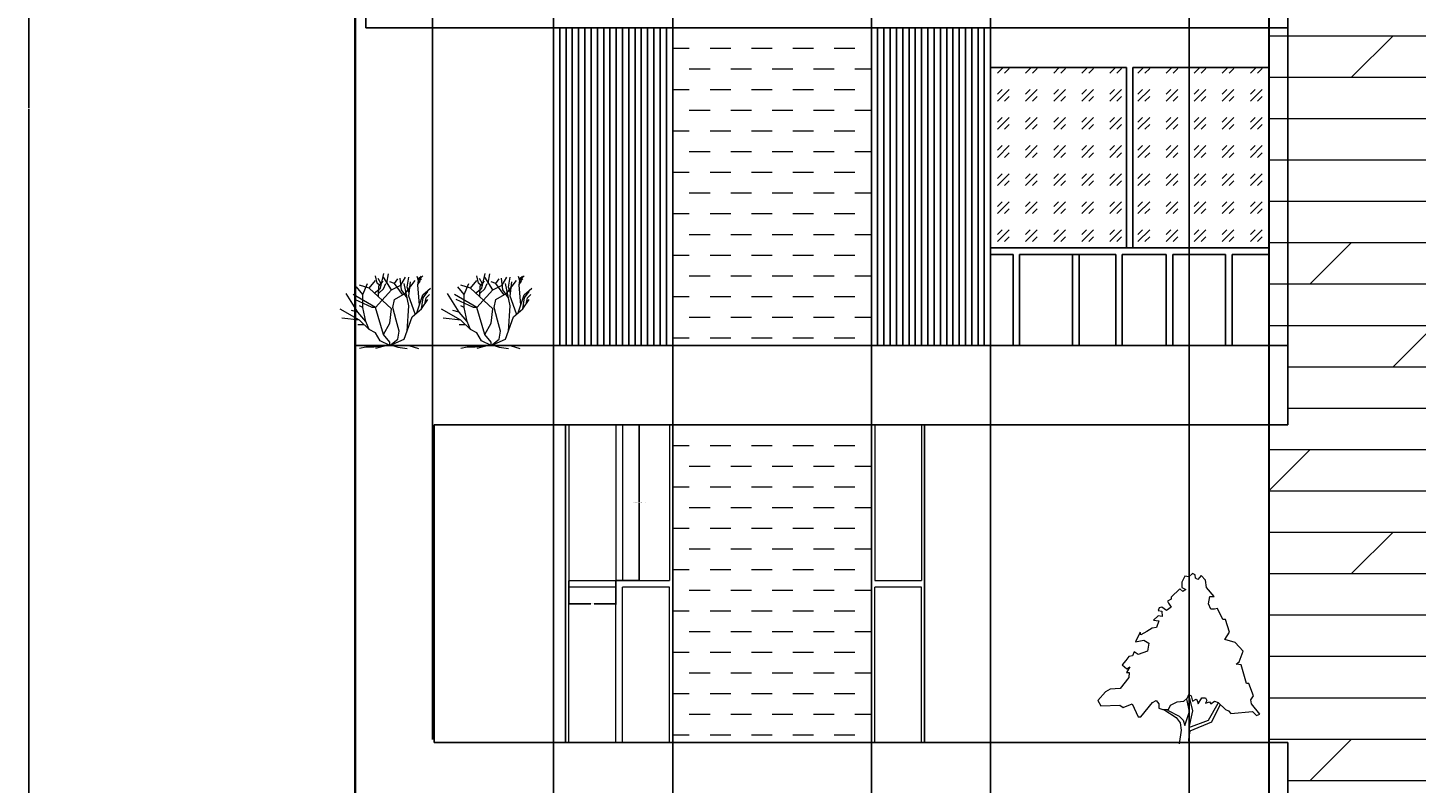
# Model space of a CAD drawing. Units: inches. Extents: x 250 to 1217, y -42 to 832.
# Tile 2 of 7: x 250 to 670, y 187 to 415. Entities that reach past the tile are written whole.
import ezdxf

# ---------------------------------------------------------------- set-up
doc = ezdxf.new("R2010")
doc.units = ezdxf.units.IN
doc.header["$MEASUREMENT"] = 0
for name, color, linetype, lineweight in [('A-ANNO-DIMS', 2, 'Continuous', 18), ('A-ELEV', 7, 'Continuous', 25), ('A-ELEV-PATT', 8, 'Continuous', 13), ('A-GLAZ', 4, 'Continuous', 18), ('L-PLNT', 3, 'Continuous', 13)]:
    doc.layers.add(name, color=color, linetype=linetype, lineweight=lineweight)
doc.styles.get("Standard").update_dxf_attribs({"font": 'arial.ttf'})
doc.dimstyles.get("Standard").update_dxf_attribs({"dimtxt": 0.18, "dimasz": 0.18, "dimexe": 0.18, "dimexo": 0.0625, "dimgap": 0.09, "dimtad": 0, "dimtih": 1, "dimtoh": 1, "dimdec": 4, "dimzin": 0, "dimdsep": 46, "dimtxsty": 'Standard', "dimcen": 0.09, "dimadec": 0, "dimazin": 0, "dimtfac": 1, "dimtdec": 4, "dimtofl": 0, "dimtmove": 0, "dimatfit": 3, "dimfxl": 1, "dimtolj": 1, "dimtzin": 0, "dimarcsym": 0})

# ---------------------------------------------------------------- blocks, each defined once
blk = doc.blocks.new('*U3')
for points in [[(22.0124, 137.721), (18.5475, 141.5624), (15.5282, 138.2446), (13.8028, 139.3505), (13.3714, 142.1153), (11.2148, 143.2214), (8.1954, 140.4564), (4.7447, 141.0094), (2.1567, 136.0326), (2.1567, 131.6088), (5.6074, 129.9499), (3.0193, 128.2909), (0.4313, 130.5029), (-6.9015, 123.3141), (-6.9015, 121.6552), (-9.9208, 119.9963), (-9.0581, 118.3373), (-6.9015, 115.0195), (-10.7835, 112.2546), (-14.6656, 115.0195), (-16.8222, 114.4665), (-17.6849, 112.2546), (-14.6656, 111.7016), (-14.2342, 107.2778), (-17.6065, 107.8307), (-21.5669, 103.9599), (-17.2536, 103.4069), (-18.9789, 97.8771), (-22.8609, 97.3241), (-27.1743, 94.5593), (-32.3504, 91.7944), (-32.7817, 94.0063), (-36.6638, 85.7116), (-29.7624, 87.3705), (-25.449, 84.6056), (-26.743, 77.9699), (-34.507, 75.205), (-37.9578, 77.4169), (-39.2518, 74.099), (-42.2711, 73.5461), (-44.8592, 70.2282), (-47.8786, 66.3574), (-43.9965, 63.0395), (-41.4085, 64.6985), (-44.3346, 59.8898), (-42.2089, 60.1377), (-42.5159, 55.7849), (-49.6039, 46.4502), (-58.2307, 45.8972), (-62.1127, 43.6853), (-68.5828, 36.4966), (-65.9947, 32.0727), (-50.0352, 32.6257), (-47.0159, 30.4138), (-39.6831, 33.7317), (-34.507, 22.6721), (-32.3504, 22.6721), (-22.4296, 34.8376), (-19.4102, 36.4966), (-17.2536, 33.7317), (-17.2536, 29.8608), (-13.8028, 28.7549), (-9.0581, 28.7549), (-7.3328, 32.6257), (-1.7254, 35.3906), (3.8821, 35.9436), (6.4701, 38.1555), (6.9014, 38.7085), (8.1954, 41.4734), (9.9208, 40.3674), (11.2148, 35.9436), (14.2341, 37.6025), (15.0968, 36.4966), (15.9595, 33.7317), (18.9789, 38.7085), (21.9982, 38.7085), (23.2922, 36.4966), (21.9982, 34.2847), (25.4489, 35.3906), (26.743, 33.7317), (29.7623, 35.9436), (32.7817, 34.8376), (38.8204, 28.7549), (41.4084, 27.6489), (43.5651, 25.437), (61.6813, 27.0959), (65.132, 23.7781), (67.7201, 24.884), (60.8186, 33.7317), (60.3873, 37.0495), (62.544, 40.3674), (58.662, 50.874), (56.5053, 50.874), (52.1919, 66.3574), (47.8785, 66.9103), (50.4665, 69.1222), (53.9172, 77.9699), (47.0158, 85.1586), (38.3891, 87.9235), (42.2711, 94.0063)], [(42.2711, 94.0063), (38.8204, 104.5129), (36.6637, 104.5129), (32.3503, 113.9135), (29.7623, 113.3605), (26.743, 113.3605), (24.5862, 117.7844), (25.8802, 123.8671), (29.331, 123.8671), (22.8609, 131.6088), (21.9982, 137.6916)], [(-9.9208, 28.2019), (0, 23.2251), (3.4507, 19.9072), (4.7447, 15.4834), (8.6267, 27.0959), (6.4701, 37.6025)], [(8.1954, 40.3674), (11.2148, 27.6489), (8.1954, 13.8245), (24.5862, 19.9072), (32.7817, 34.2847)], [(-12.9401, 28.7549), (-2.588, 22.1191), (0.8626, 17.6953), (1.7253, 11.6125), (0, 0)], [(34.5071, 33.1787), (27.1743, 18.2483), (9.0581, 10.5066), (7.7641, 3.8708), (8.1954, 0)]]:
    blk.add_lwpolyline(points)
blk = doc.blocks.new('*U2')
for p, q in [((-12.471, 19.775), (-12.898, 22.044)), ((-11.28, 19.619), (-12.104, 21.184)), ((-11.433, 18.289), (-10.457, 22.749)), ((-8.16, 17.76), (-10.56, 21.6)), ((-9.48, 19.775), (-8.992, 22.592)), ((-7.2, 19.68), (-6.24, 21.12)), ((-5.086, 17.741), (-5.513, 21.34)), ((-5.28, 19.2), (-3.84, 21.6)), ((-3.377, 18.602), (-2.888, 21.575)), ((-0.508, 21.888), (-0.081, 20.558)), ((-0.203, 19.149), (0.102, 21.34)), ((-0.02, 20.01), (0.896, 21.105)), ((0.041, 20.714), (1.384, 22.044)), ((0.102, 21.34), (0.835, 21.888)), ((-16.8, 16.32), (-18.72, 18.72)), ((-14.88, 18.24), (-17.76, 19.2)), ((-16.8, 16.32), (-15.36, 19.68)), ((-14.88, 18.24), (-12.96, 20.64)), ((-8.16, 12), (-14.88, 18.24)), ((-13.325, 16.724), (-11.433, 18.289)), ((-12.96, 12.48), (-8.16, 17.76)), ((-11.677, 19.071), (-12.471, 19.775)), ((-12.043, 15.628), (-11.921, 18.836)), ((-11.982, 16.802), (-10.579, 18.054)), ((-11.921, 18.836), (-10.64, 20.401)), ((-10.579, 18.054), (-9.846, 19.697)), ((-7.2, 19.68), (-8.64, 20.16)), ((-8.16, 17.76), (-5.28, 19.2)), ((-4.8, 16.32), (-7.2, 19.68)), ((-7.2, 14.88), (-3.84, 16.8)), ((-3.377, 15.315), (-5.086, 17.819)), ((-2.88, 12.96), (-4.32, 19.68)), ((-3.84, 16.8), (-0.96, 20.64)), ((-2.766, 16.802), (-3.377, 18.602)), ((-2.88, 15.84), (-2.4, 20.16)), ((0.346, 13.203), (-0.203, 19.149)), ((-0.142, 19.384), (0.59, 20.401)), ((1.323, 16.254), (3.642, 18.289)), ((1.44, 15.36), (2.88, 17.28)), ((-18.24, 11.04), (-21.755, 16.655)), ((-12.96, 12.48), (-19.68, 16.32)), ((-13.92, 12.48), (-19.2, 14.88)), ((-16.8, 12.48), (-17.76, 12.96)), ((-16.8, 12.48), (-16.8, 16.32)), ((-7.68, 12.48), (-7.2, 14.88)), ((-3.36, 5.28), (-2.88, 12.96)), ((-0.96, 10.56), (-2.88, 15.84)), ((-0.48, 10.8), (0.346, 13.203)), ((0.346, 13.203), (1.323, 16.254)), ((0.96, 12), (1.44, 15.36)), ((0.96, 12), (2.88, 14.88)), ((1.92, 13.44), (2.4, 15.36)), ((2.4, 15.36), (3.36, 16.32)), ((-17.76, 8.64), (-23.663, 11.961)), ((-17.76, 8.64), (-23.128, 9.222)), ((-18.24, 11.04), (-20.16, 11.52)), ((-15.84, 8.16), (-18.24, 11.04)), ((-14.88, 5.76), (-17.76, 8.64)), ((-15.84, 8.16), (-16.8, 12.48)), ((-12.96, 12.48), (-13.92, 12.48)), ((-10.56, 4.32), (-12.96, 12.48)), ((-8.64, 7.68), (-8.16, 12)), ((-6.72, 8.64), (-7.68, 12.48)), ((-5.76, 5.28), (-6.72, 8.64)), ((-4.32, 2.88), (-1.92, 9.6)), ((-1.92, 9.6), (0.96, 12)), ((-16.32, 7.2), (-18.24, 7.2)), ((-14.88, 5.76), (-15.84, 8.16)), ((-12.96, 4.8), (-14.88, 5.76)), ((-11.52, 2.4), (-12.96, 4.8)), ((-10.56, 4.32), (-8.64, 7.68)), ((-8.64, 1.92), (-10.56, 4.32)), ((-6.24, 2.88), (-5.76, 5.28)), ((-15.84, 0.48), (-17.76, 0)), ((-13.44, 0.48), (-15.84, 0.48)), ((-9.6, 0.96), (-13.44, 0.48)), ((-9.6, 0.96), (-12.96, 0)), ((-8.64, 0.96), (-11.52, 2.4)), ((-9.6, 0.96), (-7.68, 0.96)), ((-8.64, 0.96), (-4.32, 2.88)), ((-8.64, 0.96), (-6.24, 2.88)), ((-8.64, 0.96), (-8.64, 1.92)), ((-8.64, 0.96), (-2.88, 0.96)), ((-7.68, 0.96), (-6.24, 0.48)), ((-6.24, 0.48), (-3.36, 0)), ((-2.88, 0.96), (0, 0))]:
    blk.add_line(p, q)
blk = doc.blocks.new('WIN-PANEL-NARROW')
for p, q in [((0, 47), (0, 0)), ((14.16, 47), (14.16, 0)), ((0, 0), (14.16, 0))]:
    blk.add_line(p, q)
blk = doc.blocks.new('*D5')
at = {"layer": 'A-ANNO-DIMS', "color": 0, "lineweight": -2, "transparency": 16777216}
for p, q in [((427.88, 294.93), (435.05, 294.93)), ((434.87, 294.75), (434.87, 271.61)), ((434.87, 248.11), (434.87, 271.24)), ((427.88, 247.93), (435.05, 247.93))]:
    blk.add_line(p, q, dxfattribs=at)
at = {"layer": 'A-ANNO-DIMS', "color": 0, "transparency": 16777216}
for points in [[(434.84, 294.75), (434.9, 294.75), (434.87, 294.93)], [(434.84, 248.11), (434.9, 248.11), (434.87, 247.93)]]:
    blk.add_solid(points, dxfattribs=at)
at = {"layer": 'Defpoints', "color": 0, "transparency": 16777216}
for p in [(427.82, 294.93), (434.87, 294.93), (427.82, 247.93)]:
    blk.add_point(p, dxfattribs=at)
at = {"layer": 'A-ANNO-DIMS', "color": 0, "transparency": 16777216, "insert": (434.87, 271.43), "char_height": 0.18, "attachment_point": 5}
blk.add_mtext('\\A1;NARROW WINDOW PANEL 47 TYP.', dxfattribs=at)
blk = doc.blocks.new('*D6')
at = {"layer": 'A-ANNO-DIMS', "color": 0, "lineweight": -2, "transparency": 16777216}
for p, q in [((413.66, 247.86), (413.66, 240.7)), ((427.82, 247.86), (427.82, 240.7)), ((413.84, 240.88), (420.22, 240.88)), ((427.64, 240.88), (421.26, 240.88))]:
    blk.add_line(p, q, dxfattribs=at)
at = {"layer": 'A-ANNO-DIMS', "color": 0, "transparency": 16777216}
for points in [[(413.84, 240.91), (413.84, 240.85), (413.66, 240.88)], [(427.64, 240.91), (427.64, 240.85), (427.82, 240.88)]]:
    blk.add_solid(points, dxfattribs=at)
at = {"layer": 'Defpoints', "color": 0, "transparency": 16777216}
for p in [(413.66, 247.93), (427.82, 247.93), (427.82, 240.88)]:
    blk.add_point(p, dxfattribs=at)
at = {"layer": 'A-ANNO-DIMS', "color": 0, "transparency": 16777216, "insert": (420.74, 240.88), "char_height": 0.18, "attachment_point": 5}
blk.add_mtext('\\A1;14 TYP.', dxfattribs=at)
blk = doc.blocks.new('*D11')
at = {"layer": 'A-ANNO-DIMS', "color": 0, "lineweight": -2, "transparency": 16777216}
for p, q in [((352.28, 702.93), (250.36, 702.93)), ((250.54, 702.75), (250.54, 390.68)), ((250.54, 78.24), (250.54, 390.31)), ((347.84, 78.06), (250.36, 78.06))]:
    blk.add_line(p, q, dxfattribs=at)
at = {"layer": 'A-ANNO-DIMS', "color": 0, "transparency": 16777216}
for points in [[(250.51, 702.75), (250.57, 702.75), (250.54, 702.93)], [(250.51, 78.24), (250.57, 78.24), (250.54, 78.06)]]:
    blk.add_solid(points, dxfattribs=at)
at = {"layer": 'Defpoints', "color": 0, "transparency": 16777216}
for p in [(250.54, 702.93), (352.34, 702.93), (347.9, 78.06)]:
    blk.add_point(p, dxfattribs=at)
at = {"layer": 'A-ANNO-DIMS', "color": 0, "transparency": 16777216, "insert": (250.54, 390.49), "char_height": 0.18, "attachment_point": 5}
blk.add_mtext('\\A1;624.9', dxfattribs=at)
blk = doc.blocks.new('*D22')
at = {"layer": 'A-ANNO-DIMS', "color": 0, "lineweight": -2, "transparency": 16777216}
for p, q in [((349.2, 175.91), (349.2, 831.77)), ((349.38, 831.59), (378.7, 831.59)), ((408.8, 831.59), (379.49, 831.59)), ((408.98, 174.99), (408.98, 831.77))]:
    blk.add_line(p, q, dxfattribs=at)
at = {"layer": 'A-ANNO-DIMS', "color": 0, "transparency": 16777216}
for points in [[(349.38, 831.62), (349.38, 831.56), (349.2, 831.59)], [(408.8, 831.62), (408.8, 831.56), (408.98, 831.59)]]:
    blk.add_solid(points, dxfattribs=at)
at = {"layer": 'Defpoints', "color": 0, "transparency": 16777216}
for p in [(408.98, 831.59), (349.2, 175.84), (408.98, 174.93)]:
    blk.add_point(p, dxfattribs=at)
at = {"layer": 'A-ANNO-DIMS', "color": 0, "transparency": 16777216, "insert": (379.09, 831.59), "char_height": 0.18, "attachment_point": 5}
blk.add_mtext('\\A1;59.78', dxfattribs=at)
blk = doc.blocks.new('*D23')
at = {"layer": 'A-ANNO-DIMS', "color": 0, "lineweight": -2, "transparency": 16777216}
for p, q in [((408.98, 174.99), (408.98, 831.77)), ((409.16, 831.59), (426.76, 831.59)), ((444.8, 831.59), (427.2, 831.59)), ((444.98, 174.99), (444.98, 831.77))]:
    blk.add_line(p, q, dxfattribs=at)
at = {"layer": 'A-ANNO-DIMS', "color": 0, "transparency": 16777216}
for points in [[(409.16, 831.62), (409.16, 831.56), (408.98, 831.59)], [(444.8, 831.62), (444.8, 831.56), (444.98, 831.59)]]:
    blk.add_solid(points, dxfattribs=at)
at = {"layer": 'Defpoints', "color": 0, "transparency": 16777216}
for p in [(444.98, 831.59), (408.98, 174.93), (444.98, 174.93)]:
    blk.add_point(p, dxfattribs=at)
at = {"layer": 'A-ANNO-DIMS', "color": 0, "transparency": 16777216, "insert": (426.98, 831.59), "char_height": 0.18, "attachment_point": 5}
blk.add_mtext('\\A1;36', dxfattribs=at)
blk = doc.blocks.new('*D24')
at = {"layer": 'A-ANNO-DIMS', "color": 0, "lineweight": -2, "transparency": 16777216}
for p, q in [((444.98, 174.99), (444.98, 831.77)), ((445.16, 831.59), (474.76, 831.59)), ((504.8, 831.59), (475.2, 831.59)), ((504.98, 174.99), (504.98, 831.77))]:
    blk.add_line(p, q, dxfattribs=at)
at = {"layer": 'A-ANNO-DIMS', "color": 0, "transparency": 16777216}
for points in [[(445.16, 831.62), (445.16, 831.56), (444.98, 831.59)], [(504.8, 831.62), (504.8, 831.56), (504.98, 831.59)]]:
    blk.add_solid(points, dxfattribs=at)
at = {"layer": 'Defpoints', "color": 0, "transparency": 16777216}
for p in [(504.98, 831.59), (444.98, 174.93), (504.98, 174.93)]:
    blk.add_point(p, dxfattribs=at)
at = {"layer": 'A-ANNO-DIMS', "color": 0, "transparency": 16777216, "insert": (474.98, 831.59), "char_height": 0.18, "attachment_point": 5}
blk.add_mtext('\\A1;60', dxfattribs=at)
blk = doc.blocks.new('*D25')
at = {"layer": 'A-ANNO-DIMS', "color": 0, "lineweight": -2, "transparency": 16777216}
for p, q in [((504.98, 174.99), (504.98, 831.77)), ((505.16, 831.59), (522.76, 831.59)), ((540.8, 831.59), (523.2, 831.59)), ((540.98, 174.99), (540.98, 831.77))]:
    blk.add_line(p, q, dxfattribs=at)
at = {"layer": 'A-ANNO-DIMS', "color": 0, "transparency": 16777216}
for points in [[(505.16, 831.62), (505.16, 831.56), (504.98, 831.59)], [(540.8, 831.62), (540.8, 831.56), (540.98, 831.59)]]:
    blk.add_solid(points, dxfattribs=at)
at = {"layer": 'Defpoints', "color": 0, "transparency": 16777216}
for p in [(540.98, 831.59), (504.98, 174.93), (540.98, 174.93)]:
    blk.add_point(p, dxfattribs=at)
at = {"layer": 'A-ANNO-DIMS', "color": 0, "transparency": 16777216, "insert": (522.98, 831.59), "char_height": 0.18, "attachment_point": 5}
blk.add_mtext('\\A1;36', dxfattribs=at)
blk = doc.blocks.new('*D26')
at = {"layer": 'A-ANNO-DIMS', "color": 0, "lineweight": -2, "transparency": 16777216}
for p, q in [((540.98, 174.99), (540.98, 831.77)), ((541.16, 831.59), (582.76, 831.59)), ((624.8, 831.59), (583.2, 831.59)), ((624.98, 174.99), (624.98, 831.77))]:
    blk.add_line(p, q, dxfattribs=at)
at = {"layer": 'A-ANNO-DIMS', "color": 0, "transparency": 16777216}
for points in [[(541.16, 831.62), (541.16, 831.56), (540.98, 831.59)], [(624.8, 831.62), (624.8, 831.56), (624.98, 831.59)]]:
    blk.add_solid(points, dxfattribs=at)
at = {"layer": 'Defpoints', "color": 0, "transparency": 16777216}
for p in [(624.98, 831.59), (540.98, 174.93), (624.98, 174.93)]:
    blk.add_point(p, dxfattribs=at)
at = {"layer": 'A-ANNO-DIMS', "color": 0, "transparency": 16777216, "insert": (582.98, 831.59), "char_height": 0.18, "attachment_point": 5}
blk.add_mtext('\\A1;84', dxfattribs=at)
blk = doc.blocks.new('*D27')
at = {"layer": 'A-ANNO-DIMS', "color": 0, "lineweight": -2, "transparency": 16777216}
for p, q in [((624.98, 174.99), (624.98, 831.77)), ((625.16, 831.59), (655.07, 831.59)), ((685.76, 831.59), (655.86, 831.59)), ((685.94, 176.49), (685.94, 831.77))]:
    blk.add_line(p, q, dxfattribs=at)
at = {"layer": 'A-ANNO-DIMS', "color": 0, "transparency": 16777216}
for points in [[(625.16, 831.62), (625.16, 831.56), (624.98, 831.59)], [(685.76, 831.62), (685.76, 831.56), (685.94, 831.59)]]:
    blk.add_solid(points, dxfattribs=at)
at = {"layer": 'Defpoints', "color": 0, "transparency": 16777216}
for p in [(685.94, 831.59), (685.94, 176.43), (624.98, 174.93)]:
    blk.add_point(p, dxfattribs=at)
at = {"layer": 'A-ANNO-DIMS', "color": 0, "transparency": 16777216, "insert": (655.46, 831.59), "char_height": 0.18, "attachment_point": 5}
blk.add_mtext('\\A1;60.96', dxfattribs=at)
blk = doc.blocks.new('*D49')
at = {"layer": 'A-ANNO-DIMS', "color": 0, "lineweight": -2, "transparency": 16777216}
for p, q in [((348.98, 318.99), (348.98, 831.77)), ((349.16, 831.59), (489.48, 831.59)), ((630.6, 831.59), (490.28, 831.59)), ((630.78, 318.99), (630.78, 831.77))]:
    blk.add_line(p, q, dxfattribs=at)
at = {"layer": 'A-ANNO-DIMS', "color": 0, "transparency": 16777216}
for points in [[(349.16, 831.62), (349.16, 831.56), (348.98, 831.59)], [(630.6, 831.62), (630.6, 831.56), (630.78, 831.59)]]:
    blk.add_solid(points, dxfattribs=at)
at = {"layer": 'Defpoints', "color": 0, "transparency": 16777216}
for p in [(630.78, 831.59), (348.98, 318.93), (630.78, 318.93)]:
    blk.add_point(p, dxfattribs=at)
at = {"layer": 'A-ANNO-DIMS', "color": 0, "transparency": 16777216, "insert": (489.88, 831.59), "char_height": 0.18, "attachment_point": 5}
blk.add_mtext('\\A1;281.8', dxfattribs=at)
blk = doc.blocks.new('*D51')
at = {"layer": 'A-ANNO-DIMS', "color": 0, "lineweight": -2, "transparency": 16777216}
for p, q in [((348.98, 198.99), (348.98, 831.77)), ((349.16, 831.59), (360.27, 831.59)), ((372.3, 831.59), (361.2, 831.59)), ((372.48, 199.88), (372.48, 831.77))]:
    blk.add_line(p, q, dxfattribs=at)
at = {"layer": 'A-ANNO-DIMS', "color": 0, "transparency": 16777216}
for points in [[(349.16, 831.62), (349.16, 831.56), (348.98, 831.59)], [(372.3, 831.62), (372.3, 831.56), (372.48, 831.59)]]:
    blk.add_solid(points, dxfattribs=at)
at = {"layer": 'Defpoints', "color": 0, "transparency": 16777216}
for p in [(372.48, 831.59), (348.98, 198.93), (372.48, 199.81)]:
    blk.add_point(p, dxfattribs=at)
at = {"layer": 'A-ANNO-DIMS', "color": 0, "transparency": 16777216, "insert": (360.73, 831.59), "char_height": 0.18, "attachment_point": 5}
blk.add_mtext('\\A1;23.496', dxfattribs=at)
blk = doc.blocks.new('*D95')
at = {"layer": 'A-ANNO-DIMS', "color": 0, "lineweight": -2, "transparency": 16777216}
for p, q in [((625.06, 582.86), (625.06, -41.6)), ((600.97, 582.52), (600.97, -41.6)), ((601.15, -41.42), (612.62, -41.42)), ((624.88, -41.42), (613.41, -41.42))]:
    blk.add_line(p, q, dxfattribs=at)
at = {"layer": 'A-ANNO-DIMS', "color": 0, "transparency": 16777216}
for points in [[(601.15, -41.39), (601.15, -41.45), (600.97, -41.42)], [(624.88, -41.39), (624.88, -41.45), (625.06, -41.42)]]:
    blk.add_solid(points, dxfattribs=at)
at = {"layer": 'Defpoints', "color": 0, "transparency": 16777216}
for p in [(625.06, 582.93), (600.97, 582.58), (625.06, -41.42)]:
    blk.add_point(p, dxfattribs=at)
at = {"layer": 'A-ANNO-DIMS', "color": 0, "transparency": 16777216, "insert": (613.02, -41.42), "char_height": 0.18, "attachment_point": 5}
blk.add_mtext('\\A1;24.10', dxfattribs=at)

msp = doc.modelspace()

# ---------------------------------------------------------------- hatches: boundary and pattern name
at = {"layer": 'A-ELEV-PATT'}
h = msp.add_hatch(dxfattribs=at)
h.set_pattern_fill('DOLMIT', color=256, scale=50)
h.paths.add_polyline_path([(684.9826, 558.9271), (679.1872, 558.9271), (679.1872, 582.9271), (685.0649, 582.9271), (685.0649, 678.9271), (679.1872, 678.9271), (679.1872, 702.9271), (630.7779, 702.9271), (630.7779, 678.9271), (625.0649, 678.9271), (625.0649, 582.9271), (630.7779, 582.9271), (630.7779, 558.9271), (624.9826, 558.9271), (624.9826, 438.9271), (630.7779, 438.9271), (630.7779, 414.9271), (624.9826, 414.9271), (624.9826, 318.9271), (630.7779, 318.9271), (630.7779, 294.9271), (624.9826, 294.9271), (624.9826, 198.9271), (630.7779, 198.9271), (630.7779, 174.9271), (624.9826, 174.9271), (624.9826, 78.9271), (684.9826, 78.9271), (684.9826, 174.9271), (679.1872, 174.9271), (679.1872, 198.9271), (683.6004, 198.9271), (684.9826, 198.9271), (684.9826, 294.9271), (679.1872, 294.9271), (679.1872, 318.9271), (684.9826, 318.9271), (684.9826, 414.9271), (679.1872, 414.9271), (679.1872, 438.9271), (684.9826, 438.9271)])
h = msp.add_hatch(dxfattribs=at)
h.set_pattern_fill('DASH', color=256, scale=50)
h.set_pattern_definition([(0, (0, 240), (6.25, 6.25), [6.25, -6.25])])
h.paths.add_polyline_path([(504.9826, 414.9271), (444.9826, 414.9271), (444.9826, 318.9271), (504.9826, 318.9271)])
h = msp.add_hatch(dxfattribs=at)
h.set_pattern_fill('GOST_GLASS', color=256)
h.set_pattern_definition([(45, (0, 240), (8.48528, 0), [5, -7]), (45, (2.1213, 240), (8.48528, 0), [2, -10]), (45, (0, 242.1213), (8.48528, 0), [2, -10])])
h.paths.add_polyline_path([(581.9826, 402.9271), (540.9826, 402.9271), (540.9826, 348.4651), (578.7563, 348.4651), (581.9826, 348.4651)])
h.paths.add_polyline_path([(624.9826, 402.9271), (583.9826, 402.9271), (583.9826, 348.4651), (624.9826, 348.4651)])
h = msp.add_hatch(dxfattribs=at)
h.set_pattern_fill('DASH', color=256, scale=50)
h.set_pattern_definition([(0, (0, 120), (6.25, 6.25), [6.25, -6.25])])
h.paths.add_polyline_path([(504.9826, 294.9271), (444.9826, 294.9271), (444.9826, 198.9271), (504.9826, 198.9271)])

# ---------------------------------------------------------------- linework, layer by layer
at = {"layer": 'A-ELEV'}
for p, q in [((352.3429, 414.9271), (352.3429, 438.9271)), ((352.3429, 414.9271), (630.7779, 414.9271)), ((408.9826, 414.9271), (408.9826, 318.9271)), ((408.9826, 414.9271), (630.7779, 414.9271)), ((410.8773, 414.9271), (410.8773, 318.9271)), ((412.772, 414.9271), (412.772, 318.9271)), ((414.6668, 414.9271), (414.6668, 318.9271)), ((416.5615, 414.9271), (416.5615, 318.9271)), ((418.4563, 414.9271), (418.4563, 318.9271)), ((420.351, 414.9271), (420.351, 318.9271)), ((422.2457, 414.9271), (422.2457, 318.9271)), ((424.1405, 414.9271), (424.1405, 318.9271)), ((426.0352, 414.9271), (426.0352, 318.9271)), ((427.9299, 414.9271), (427.9299, 318.9271)), ((429.8247, 414.9271), (429.8247, 318.9271)), ((431.7194, 414.9271), (431.7194, 318.9271)), ((433.6142, 414.9271), (433.6142, 318.9271)), ((435.5089, 414.9271), (435.5089, 318.9271)), ((437.4036, 414.9271), (437.4036, 318.9271)), ((439.2984, 414.9271), (439.2984, 318.9271)), ((441.1931, 414.9271), (441.1931, 318.9271)), ((443.0878, 414.9271), (443.0878, 318.9271)), ((444.9826, 414.9271), (444.9826, 318.9271)), ((444.9826, 414.9271), (444.9826, 318.9271)), ((444.9826, 414.9271), (444.9826, 318.9271)), ((444.9826, 414.9271), (444.9826, 318.9271)), ((504.9826, 414.9271), (504.9826, 318.9271)), ((506.8773, 414.9271), (506.8773, 318.9271)), ((508.772, 414.9271), (508.772, 318.9271)), ((510.6668, 414.9271), (510.6668, 318.9271)), ((512.5615, 414.9271), (512.5615, 318.9271)), ((514.4563, 414.9271), (514.4563, 318.9271)), ((516.351, 414.9271), (516.351, 318.9271)), ((518.2457, 414.9271), (518.2457, 318.9271)), ((520.1405, 414.9271), (520.1405, 318.9271)), ((522.0352, 414.9271), (522.0352, 318.9271)), ((523.9299, 414.9271), (523.9299, 318.9271)), ((525.8247, 414.9271), (525.8247, 318.9271)), ((527.7194, 414.9271), (527.7194, 318.9271)), ((529.6142, 414.9271), (529.6142, 318.9271)), ((531.5089, 414.9271), (531.5089, 318.9271)), ((533.4036, 414.9271), (533.4036, 318.9271)), ((535.2984, 414.9271), (535.2984, 318.9271)), ((537.1931, 414.9271), (537.1931, 318.9271)), ((539.0878, 414.9271), (539.0878, 318.9271)), ((540.9826, 414.9271), (540.9826, 318.9271)), ((624.9826, 414.9271), (624.9826, 318.9271)), ((581.9826, 402.9271), (540.9826, 402.9271)), ((581.9826, 402.9271), (581.9826, 348.4651)), ((583.9826, 402.9271), (583.9826, 348.4651)), ((583.9826, 402.9271), (624.9826, 402.9271)), ((624.9826, 402.9271), (583.9826, 402.9271)), ((578.7563, 348.4651), (540.9826, 348.4651)), ((624.9826, 348.4651), (564.9826, 348.4651)), ((547.7563, 346.4651), (540.9826, 346.4651)), ((547.7563, 346.4651), (547.7563, 318.9271)), ((549.7563, 346.4651), (549.7563, 318.9271)), ((565.684, 346.4651), (549.7563, 346.4651)), ((578.7563, 346.4651), (564.9826, 346.4651)), ((565.684, 346.4651), (565.684, 318.9271)), ((578.7563, 346.4651), (567.684, 346.4651)), ((567.684, 346.4651), (567.684, 318.9271)), ((578.7563, 346.4651), (578.7563, 318.9271)), ((593.9826, 346.4651), (580.7563, 346.4651)), ((580.7563, 346.4651), (580.7563, 318.9271)), ((593.9826, 346.4651), (593.9826, 318.9271)), ((595.9826, 346.4651), (595.9826, 318.9271)), ((611.9103, 346.4651), (595.9826, 346.4651)), ((611.9103, 346.4651), (611.9103, 318.9271)), ((624.9826, 346.4651), (613.9103, 346.4651)), ((613.9103, 346.4651), (613.9103, 318.9271)), ((348.9826, 318.9271), (630.7779, 318.9271)), ((630.7779, 318.9271), (630.7779, 294.9271)), ((412.6561, 294.9271), (412.6561, 198.9271)), ((412.6561, 294.9271), (412.6561, 198.9271)), ((412.6561, 294.9271), (412.6561, 198.9271)), ((412.6561, 294.9271), (412.6561, 198.9271)), ((444.9826, 294.9271), (444.9826, 198.9271)), ((444.9826, 294.9271), (444.9826, 198.9271)), ((444.9826, 294.9271), (444.9826, 198.9271)), ((444.9826, 294.9271), (444.9826, 198.9271)), ((504.9826, 294.9271), (504.9826, 198.9271)), ((504.9826, 294.9271), (504.9826, 198.9271)), ((504.9826, 294.9271), (504.9826, 198.9271)), ((504.9826, 294.9271), (504.9826, 198.9271)), ((504.9826, 294.9271), (504.9826, 198.9271)), ((520.9846, 198.9271), (520.9846, 294.9271)), ((624.9826, 294.9271), (624.9826, 198.9271)), ((348.9826, 198.9271), (348.9826, 174.9271)), ((372.9826, 198.9271), (630.7779, 198.9271)), ((630.7779, 198.9271), (372.9826, 198.9271)), ((630.7779, 198.9271), (630.7779, 174.9271))]:
    msp.add_line(p, q, dxfattribs=at)
for points in [[(630.7779, 318.9271), (348.9826, 318.9271), (348.9826, 198.9271)], [(630.7779, 294.9271), (372.9826, 294.9271), (372.9826, 198.9271)]]:
    msp.add_lwpolyline(points, dxfattribs=at)

# ---------------------------------------------------------------- block references
at = {"layer": 'A-GLAZ'}
for p in [(413.656, 247.927), (429.8192, 247.927), (505.9824, 247.927)]:
    msp.add_blockref('WIN-PANEL-NARROW', p, dxfattribs=at)
at = {"layer": 'A-GLAZ', "rotation": 180}
for p in [(427.8195, 245.9271), (443.9827, 245.9271), (520.1459, 245.9271)]:
    msp.add_blockref('WIN-PANEL-NARROW', p, dxfattribs=at)
at = {"layer": 'L-PLNT'}
for p in [(368.1829, 317.9671), (398.7837, 317.9671)]:
    msp.add_blockref('*U2', p, dxfattribs=at)
at = {"layer": 'L-PLNT', "xscale": 0.3589292991008459, "yscale": 0.3589292991008459, "zscale": 0.3589292991008459}
msp.add_blockref('*U3', (597.9433, 198.5825), dxfattribs=at)

# ---------------------------------------------------------------- dimensions: what is measured, and where the dimension line sits
at = {"layer": 'A-ANNO-DIMS'}
for base, p1, p2, override, picture, middle in [((630.7779, 831.5941), (348.9826, 318.9271), (630.7779, 318.9271), {"dimdec": 1, "dimlfac": 1, "dimrnd": 0, "dimzin": 0, "dimdsep": 46, "dimlunit": 2}, '*D49', (489.8803, 831.5941)), ((372.4789, 831.5941), (348.9826, 198.9271), (372.4789, 199.8131), {"dimdec": 3, "dimlfac": 1, "dimrnd": 0, "dimzin": 0, "dimdsep": 46, "dimlunit": 2}, '*D51', (360.7307, 831.5941)), ((408.9826, 831.5941), (349.204, 175.8442), (408.9826, 174.9271), {"dimdec": 2, "dimlfac": 1, "dimrnd": 0, "dimzin": 0, "dimdsep": 46, "dimlunit": 2}, '*D22', (379.0933, 831.5941)), ((444.9826, 831.5941), (408.9826, 174.9271), (444.9826, 174.9271), {"dimdec": 0, "dimlfac": 1, "dimrnd": 0, "dimzin": 0, "dimdsep": 46, "dimlunit": 2}, '*D23', (426.9826, 831.5941)), ((504.9826, 831.5941), (444.9826, 174.9271), (504.9826, 174.9271), {"dimdec": 0, "dimlfac": 1, "dimrnd": 0, "dimzin": 0, "dimdsep": 46, "dimlunit": 2}, '*D24', (474.9826, 831.5941)), ((540.9826, 831.5941), (504.9826, 174.9271), (540.9826, 174.9271), {"dimdec": 0, "dimlfac": 1, "dimrnd": 0, "dimzin": 0, "dimdsep": 46, "dimlunit": 2}, '*D25', (522.9826, 831.5941)), ((624.9826, 831.5941), (540.9826, 174.9271), (624.9826, 174.9271), {"dimdec": 0, "dimlfac": 1, "dimrnd": 0, "dimzin": 0, "dimdsep": 46, "dimlunit": 2}, '*D26', (582.9826, 831.5941)), ((685.944, 831.5941), (624.9826, 174.9271), (685.944, 176.4321), {"dimdec": 2, "dimlfac": 1, "dimrnd": 0, "dimzin": 0, "dimdsep": 46, "dimlunit": 2}, '*D27', (655.4633, 831.5941)), ((625.0649, -41.4199), (600.9672, 582.5825), (625.0649, 582.9271), {"dimdec": 2, "dimlfac": 1, "dimrnd": 0, "dimzin": 0, "dimdsep": 46, "dimlunit": 2}, '*D95', (613.0161, -41.4199))]:
    dim = msp.add_linear_dim(base=base, p1=p1, p2=p2, dimstyle='Standard', override=override, dxfattribs=at)
    dim.commit()
    dim.dimension.update_dxf_attribs({"geometry": picture, "text_midpoint": middle})
dim = msp.add_linear_dim(base=(250.5369, 702.9271), p1=(347.8976, 78.0612), p2=(352.3429, 702.9271), angle=90, dimstyle='Standard', override={"dimdec": 1, "dimlfac": 1, "dimrnd": 0, "dimzin": 0, "dimdsep": 46, "dimlunit": 2}, dxfattribs=at)
dim.commit()
dim.dimension.update_dxf_attribs({"geometry": '*D11', "text_midpoint": (250.5369, 390.4941)})
dim = msp.add_linear_dim(base=(434.8694, 294.9271), p1=(427.8194, 247.9271), p2=(427.8194, 294.9271), angle=90, text='NARROW WINDOW PANEL <> TYP.', dimstyle='Standard', override={"dimdec": 0, "dimlfac": 1, "dimrnd": 0, "dimzin": 0, "dimdsep": 46, "dimlunit": 2}, dxfattribs=at)
dim.commit()
dim.dimension.update_dxf_attribs({"geometry": '*D5', "text_midpoint": (434.8694, 271.4271)})
dim = msp.add_linear_dim(base=(427.8194, 240.8771), p1=(413.6561, 247.9271), p2=(427.8194, 247.9271), text='<> TYP.', dimstyle='Standard', override={"dimdec": 0, "dimlfac": 1, "dimrnd": 0, "dimzin": 0, "dimdsep": 46, "dimlunit": 2}, dxfattribs=at)
dim.commit()
dim.dimension.update_dxf_attribs({"geometry": '*D6', "text_midpoint": (420.7377, 240.8771)})

doc.saveas('drawing.dxf')
